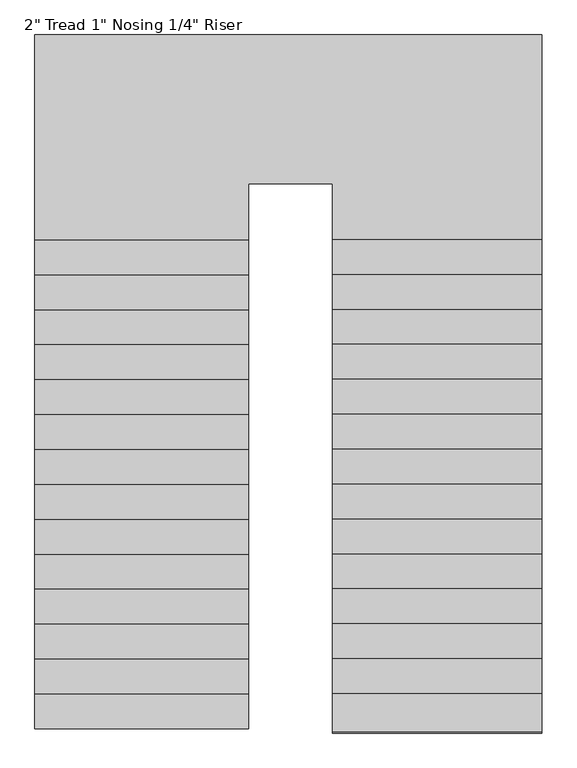
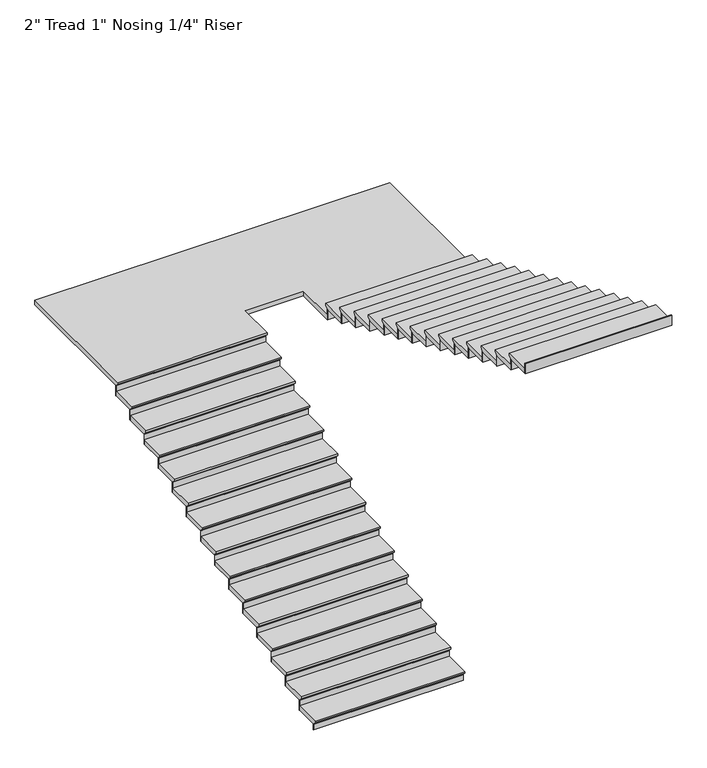
"""IFC4 building model written with IfcOpenShell, lengths in millimetres: stair flight geometry."""

from ifc_helpers import new_model, si_unit, origin, place, context, project, spatial, faceted_brep, source, transform, mapped, element, save


def stair_flight_0f889a08(model_context):
    return source(origin(), model_context, "Body", "Brep", [
        faceted_brep([(-5999.9290366, -6973.0610642, 8931.91), (-5999.9290366, -6973.0610642, 8950.96), (-7554.4415084, -6973.0610642, 8950.96), (-7554.4415084, -6973.0610642, 8931.91), (-5999.9290366, -6947.6610642, 8906.51), (-7554.4415084, -6947.6610642, 8906.51), (-5999.9290366, -6693.6610642, 8950.96), (-7554.4415084, -6693.6610642, 8950.96), (-7554.4415084, -6947.6610642, 8900.16), (-7554.4415084, -6693.6610642, 8900.16), (-5999.9290366, -6693.6610642, 8900.16), (-5999.9290366, -6947.6610642, 8900.16)], [[[0, 1, 2, 3]], [[4, 0, 3, 5]], [[2, 1, 6, 7]], [[8, 9, 10, 11]], [[2, 7, 9, 8, 5, 3]], [[8, 11, 4, 5]], [[6, 1, 0, 4, 11, 10]], [[7, 6, 10, 9]]]),
        faceted_brep([(-5999.9290366, -6947.6610642, 8900.16), (-5999.9290366, -6947.6610642, 8839.2), (-5999.9290366, -6941.3110642, 8839.2), (-5999.9290366, -6941.3110642, 8900.16), (-7554.4415084, -6947.6610642, 8900.16), (-7554.4415084, -6941.3110642, 8900.16), (-7554.4415084, -6941.3110642, 8839.2), (-7554.4415084, -6947.6610642, 8839.2)], [[[0, 1, 2, 3]], [[4, 5, 6, 7]], [[1, 0, 4, 7]], [[2, 1, 7, 6]], [[3, 2, 6, 5]], [[0, 3, 5, 4]]]),
        faceted_brep([(-5999.9290366, -6693.6610642, 9011.92), (-5999.9290366, -6693.6610642, 8900.16), (-5999.9290366, -6687.3110642, 8900.16), (-5999.9290366, -6687.3110642, 9011.92), (-7554.4415084, -6693.6610642, 9011.92), (-7554.4415084, -6687.3110642, 9011.92), (-7554.4415084, -6687.3110642, 8900.16), (-7554.4415084, -6693.6610642, 8900.16)], [[[0, 1, 2, 3]], [[4, 5, 6, 7]], [[1, 0, 4, 7]], [[2, 1, 7, 6]], [[3, 2, 6, 5]], [[0, 3, 5, 4]]]),
        faceted_brep([(-7554.4415084, -6719.0610642, 9062.72), (-5999.9290366, -6719.0610642, 9062.72), (-5999.9290366, -6439.6610642, 9062.72), (-7554.4415084, -6439.6610642, 9062.72), (-7554.4415084, -6693.6610642, 9011.92), (-7554.4415084, -6439.6610642, 9011.92), (-5999.9290366, -6439.6610642, 9011.92), (-5999.9290366, -6693.6610642, 9011.92), (-7554.4415084, -6693.6610642, 9018.27), (-7554.4415084, -6719.0610642, 9043.67), (-5999.9290366, -6693.6610642, 9018.27), (-5999.9290366, -6719.0610642, 9043.67)], [[[0, 1, 2, 3]], [[4, 5, 6, 7]], [[0, 3, 5, 4, 8, 9]], [[4, 7, 10, 8]], [[2, 1, 11, 10, 7, 6]], [[3, 2, 6, 5]], [[11, 1, 0, 9]], [[10, 11, 9, 8]]]),
        faceted_brep([(-5999.9290366, -6439.6610642, 9123.68), (-5999.9290366, -6439.6610642, 9011.92), (-5999.9290366, -6433.3110642, 9011.92), (-5999.9290366, -6433.3110642, 9123.68), (-7554.4415084, -6439.6610642, 9123.68), (-7554.4415084, -6433.3110642, 9123.68), (-7554.4415084, -6433.3110642, 9011.92), (-7554.4415084, -6439.6610642, 9011.92)], [[[0, 1, 2, 3]], [[4, 5, 6, 7]], [[1, 0, 4, 7]], [[2, 1, 7, 6]], [[3, 2, 6, 5]], [[0, 3, 5, 4]]]),
        faceted_brep([(-7554.4415084, -6465.0610642, 9174.48), (-5999.9290366, -6465.0610642, 9174.48), (-5999.9290366, -6185.6610642, 9174.48), (-7554.4415084, -6185.6610642, 9174.48), (-7554.4415084, -6439.6610642, 9123.68), (-7554.4415084, -6185.6610642, 9123.68), (-5999.9290366, -6185.6610642, 9123.68), (-5999.9290366, -6439.6610642, 9123.68), (-7554.4415084, -6439.6610642, 9130.03), (-7554.4415084, -6465.0610642, 9155.43), (-5999.9290366, -6439.6610642, 9130.03), (-5999.9290366, -6465.0610642, 9155.43)], [[[0, 1, 2, 3]], [[4, 5, 6, 7]], [[0, 3, 5, 4, 8, 9]], [[4, 7, 10, 8]], [[2, 1, 11, 10, 7, 6]], [[3, 2, 6, 5]], [[11, 1, 0, 9]], [[10, 11, 9, 8]]]),
        faceted_brep([(-5999.9290366, -6185.6610642, 9235.44), (-5999.9290366, -6185.6610642, 9123.68), (-5999.9290366, -6179.3110642, 9123.68), (-5999.9290366, -6179.3110642, 9235.44), (-7554.4415084, -6185.6610642, 9235.44), (-7554.4415084, -6179.3110642, 9235.44), (-7554.4415084, -6179.3110642, 9123.68), (-7554.4415084, -6185.6610642, 9123.68)], [[[0, 1, 2, 3]], [[4, 5, 6, 7]], [[1, 0, 4, 7]], [[2, 1, 7, 6]], [[3, 2, 6, 5]], [[0, 3, 5, 4]]]),
        faceted_brep([(-7554.4415084, -6211.0610642, 9286.24), (-5999.9290366, -6211.0610642, 9286.24), (-5999.9290366, -5931.6610642, 9286.24), (-7554.4415084, -5931.6610642, 9286.24), (-7554.4415084, -6185.6610642, 9235.44), (-7554.4415084, -5931.6610642, 9235.44), (-5999.9290366, -5931.6610642, 9235.44), (-5999.9290366, -6185.6610642, 9235.44), (-7554.4415084, -6185.6610642, 9241.79), (-7554.4415084, -6211.0610642, 9267.19), (-5999.9290366, -6185.6610642, 9241.79), (-5999.9290366, -6211.0610642, 9267.19)], [[[0, 1, 2, 3]], [[4, 5, 6, 7]], [[0, 3, 5, 4, 8, 9]], [[4, 7, 10, 8]], [[2, 1, 11, 10, 7, 6]], [[3, 2, 6, 5]], [[11, 1, 0, 9]], [[10, 11, 9, 8]]]),
        faceted_brep([(-5999.9290366, -5931.6610642, 9347.2), (-5999.9290366, -5931.6610642, 9235.44), (-5999.9290366, -5925.3110642, 9235.44), (-5999.9290366, -5925.3110642, 9347.2), (-7554.4415084, -5931.6610642, 9347.2), (-7554.4415084, -5925.3110642, 9347.2), (-7554.4415084, -5925.3110642, 9235.44), (-7554.4415084, -5931.6610642, 9235.44)], [[[0, 1, 2, 3]], [[4, 5, 6, 7]], [[1, 0, 4, 7]], [[2, 1, 7, 6]], [[3, 2, 6, 5]], [[0, 3, 5, 4]]]),
        faceted_brep([(-7554.4415084, -5957.0610642, 9398.0), (-5999.9290366, -5957.0610642, 9398.0), (-5999.9290366, -5677.6610642, 9398.0), (-7554.4415084, -5677.6610642, 9398.0), (-7554.4415084, -5931.6610642, 9347.2), (-7554.4415084, -5677.6610642, 9347.2), (-5999.9290366, -5677.6610642, 9347.2), (-5999.9290366, -5931.6610642, 9347.2), (-7554.4415084, -5931.6610642, 9353.55), (-7554.4415084, -5957.0610642, 9378.95), (-5999.9290366, -5931.6610642, 9353.55), (-5999.9290366, -5957.0610642, 9378.95)], [[[0, 1, 2, 3]], [[4, 5, 6, 7]], [[0, 3, 5, 4, 8, 9]], [[4, 7, 10, 8]], [[2, 1, 11, 10, 7, 6]], [[3, 2, 6, 5]], [[11, 1, 0, 9]], [[10, 11, 9, 8]]]),
        faceted_brep([(-5999.9290366, -5677.6610642, 9458.96), (-5999.9290366, -5677.6610642, 9347.2), (-5999.9290366, -5671.3110642, 9347.2), (-5999.9290366, -5671.3110642, 9458.96), (-7554.4415084, -5677.6610642, 9458.96), (-7554.4415084, -5671.3110642, 9458.96), (-7554.4415084, -5671.3110642, 9347.2), (-7554.4415084, -5677.6610642, 9347.2)], [[[0, 1, 2, 3]], [[4, 5, 6, 7]], [[1, 0, 4, 7]], [[2, 1, 7, 6]], [[3, 2, 6, 5]], [[0, 3, 5, 4]]]),
        faceted_brep([(-7554.4415084, -5703.0610642, 9509.76), (-5999.9290366, -5703.0610642, 9509.76), (-5999.9290366, -5423.6610642, 9509.76), (-7554.4415084, -5423.6610642, 9509.76), (-7554.4415084, -5677.6610642, 9458.96), (-7554.4415084, -5423.6610642, 9458.96), (-5999.9290366, -5423.6610642, 9458.96), (-5999.9290366, -5677.6610642, 9458.96), (-7554.4415084, -5677.6610642, 9465.31), (-7554.4415084, -5703.0610642, 9490.71), (-5999.9290366, -5677.6610642, 9465.31), (-5999.9290366, -5703.0610642, 9490.71)], [[[0, 1, 2, 3]], [[4, 5, 6, 7]], [[0, 3, 5, 4, 8, 9]], [[4, 7, 10, 8]], [[2, 1, 11, 10, 7, 6]], [[3, 2, 6, 5]], [[11, 1, 0, 9]], [[10, 11, 9, 8]]]),
        faceted_brep([(-5999.9290366, -5423.6610642, 9570.72), (-5999.9290366, -5423.6610642, 9458.96), (-5999.9290366, -5417.3110642, 9458.96), (-5999.9290366, -5417.3110642, 9570.72), (-7554.4415084, -5423.6610642, 9570.72), (-7554.4415084, -5417.3110642, 9570.72), (-7554.4415084, -5417.3110642, 9458.96), (-7554.4415084, -5423.6610642, 9458.96)], [[[0, 1, 2, 3]], [[4, 5, 6, 7]], [[1, 0, 4, 7]], [[2, 1, 7, 6]], [[3, 2, 6, 5]], [[0, 3, 5, 4]]]),
        faceted_brep([(-7554.4415084, -5449.0610642, 9621.52), (-5999.9290366, -5449.0610642, 9621.52), (-5999.9290366, -5169.6610642, 9621.52), (-7554.4415084, -5169.6610642, 9621.52), (-7554.4415084, -5423.6610642, 9570.72), (-7554.4415084, -5169.6610642, 9570.72), (-5999.9290366, -5169.6610642, 9570.72), (-5999.9290366, -5423.6610642, 9570.72), (-7554.4415084, -5423.6610642, 9577.07), (-7554.4415084, -5449.0610642, 9602.47), (-5999.9290366, -5423.6610642, 9577.07), (-5999.9290366, -5449.0610642, 9602.47)], [[[0, 1, 2, 3]], [[4, 5, 6, 7]], [[0, 3, 5, 4, 8, 9]], [[4, 7, 10, 8]], [[2, 1, 11, 10, 7, 6]], [[3, 2, 6, 5]], [[11, 1, 0, 9]], [[10, 11, 9, 8]]]),
        faceted_brep([(-5999.9290366, -5169.6610642, 9682.48), (-5999.9290366, -5169.6610642, 9570.72), (-5999.9290366, -5163.3110642, 9570.72), (-5999.9290366, -5163.3110642, 9682.48), (-7554.4415084, -5169.6610642, 9682.48), (-7554.4415084, -5163.3110642, 9682.48), (-7554.4415084, -5163.3110642, 9570.72), (-7554.4415084, -5169.6610642, 9570.72)], [[[0, 1, 2, 3]], [[4, 5, 6, 7]], [[1, 0, 4, 7]], [[2, 1, 7, 6]], [[3, 2, 6, 5]], [[0, 3, 5, 4]]]),
        faceted_brep([(-7554.4415084, -5195.0610642, 9733.28), (-5999.9290366, -5195.0610642, 9733.28), (-5999.9290366, -4915.6610642, 9733.28), (-7554.4415084, -4915.6610642, 9733.28), (-7554.4415084, -5169.6610642, 9682.48), (-7554.4415084, -4915.6610642, 9682.48), (-5999.9290366, -4915.6610642, 9682.48), (-5999.9290366, -5169.6610642, 9682.48), (-7554.4415084, -5169.6610642, 9688.83), (-7554.4415084, -5195.0610642, 9714.23), (-5999.9290366, -5169.6610642, 9688.83), (-5999.9290366, -5195.0610642, 9714.23)], [[[0, 1, 2, 3]], [[4, 5, 6, 7]], [[0, 3, 5, 4, 8, 9]], [[4, 7, 10, 8]], [[2, 1, 11, 10, 7, 6]], [[3, 2, 6, 5]], [[11, 1, 0, 9]], [[10, 11, 9, 8]]]),
        faceted_brep([(-5999.9290366, -4915.6610642, 9794.24), (-5999.9290366, -4915.6610642, 9682.48), (-5999.9290366, -4909.3110642, 9682.48), (-5999.9290366, -4909.3110642, 9794.24), (-7554.4415084, -4915.6610642, 9794.24), (-7554.4415084, -4909.3110642, 9794.24), (-7554.4415084, -4909.3110642, 9682.48), (-7554.4415084, -4915.6610642, 9682.48)], [[[0, 1, 2, 3]], [[4, 5, 6, 7]], [[1, 0, 4, 7]], [[2, 1, 7, 6]], [[3, 2, 6, 5]], [[0, 3, 5, 4]]]),
        faceted_brep([(-7554.4415084, -4941.0610642, 9845.04), (-5999.9290366, -4941.0610642, 9845.04), (-5999.9290366, -4661.6610642, 9845.04), (-7554.4415084, -4661.6610642, 9845.04), (-7554.4415084, -4915.6610642, 9794.24), (-7554.4415084, -4661.6610642, 9794.24), (-5999.9290366, -4661.6610642, 9794.24), (-5999.9290366, -4915.6610642, 9794.24), (-7554.4415084, -4915.6610642, 9800.59), (-7554.4415084, -4941.0610642, 9825.99), (-5999.9290366, -4915.6610642, 9800.59), (-5999.9290366, -4941.0610642, 9825.99)], [[[0, 1, 2, 3]], [[4, 5, 6, 7]], [[0, 3, 5, 4, 8, 9]], [[4, 7, 10, 8]], [[2, 1, 11, 10, 7, 6]], [[3, 2, 6, 5]], [[11, 1, 0, 9]], [[10, 11, 9, 8]]]),
        faceted_brep([(-5999.9290366, -4661.6610642, 9906.0), (-5999.9290366, -4661.6610642, 9794.24), (-5999.9290366, -4655.3110642, 9794.24), (-5999.9290366, -4655.3110642, 9906.0), (-7554.4415084, -4661.6610642, 9906.0), (-7554.4415084, -4655.3110642, 9906.0), (-7554.4415084, -4655.3110642, 9794.24), (-7554.4415084, -4661.6610642, 9794.24)], [[[0, 1, 2, 3]], [[4, 5, 6, 7]], [[1, 0, 4, 7]], [[2, 1, 7, 6]], [[3, 2, 6, 5]], [[0, 3, 5, 4]]]),
        faceted_brep([(-7554.4415084, -4687.0610642, 9956.8), (-5999.9290366, -4687.0610642, 9956.8), (-5999.9290366, -4407.6610642, 9956.8), (-7554.4415084, -4407.6610642, 9956.8), (-7554.4415084, -4661.6610642, 9906.0), (-7554.4415084, -4407.6610642, 9906.0), (-5999.9290366, -4407.6610642, 9906.0), (-5999.9290366, -4661.6610642, 9906.0), (-7554.4415084, -4661.6610642, 9912.35), (-7554.4415084, -4687.0610642, 9937.75), (-5999.9290366, -4661.6610642, 9912.35), (-5999.9290366, -4687.0610642, 9937.75)], [[[0, 1, 2, 3]], [[4, 5, 6, 7]], [[0, 3, 5, 4, 8, 9]], [[4, 7, 10, 8]], [[2, 1, 11, 10, 7, 6]], [[3, 2, 6, 5]], [[11, 1, 0, 9]], [[10, 11, 9, 8]]]),
        faceted_brep([(-5999.9290366, -4407.6610642, 10017.76), (-5999.9290366, -4407.6610642, 9906.0), (-5999.9290366, -4401.3110642, 9906.0), (-5999.9290366, -4401.3110642, 10017.76), (-7554.4415084, -4407.6610642, 10017.76), (-7554.4415084, -4401.3110642, 10017.76), (-7554.4415084, -4401.3110642, 9906.0), (-7554.4415084, -4407.6610642, 9906.0)], [[[0, 1, 2, 3]], [[4, 5, 6, 7]], [[1, 0, 4, 7]], [[2, 1, 7, 6]], [[3, 2, 6, 5]], [[0, 3, 5, 4]]]),
        faceted_brep([(-7554.4415084, -4433.0610642, 10068.56), (-5999.9290366, -4433.0610642, 10068.56), (-5999.9290366, -4153.6610642, 10068.56), (-7554.4415084, -4153.6610642, 10068.56), (-7554.4415084, -4407.6610642, 10017.76), (-7554.4415084, -4153.6610642, 10017.76), (-5999.9290366, -4153.6610642, 10017.76), (-5999.9290366, -4407.6610642, 10017.76), (-7554.4415084, -4407.6610642, 10024.11), (-7554.4415084, -4433.0610642, 10049.51), (-5999.9290366, -4407.6610642, 10024.11), (-5999.9290366, -4433.0610642, 10049.51)], [[[0, 1, 2, 3]], [[4, 5, 6, 7]], [[0, 3, 5, 4, 8, 9]], [[4, 7, 10, 8]], [[2, 1, 11, 10, 7, 6]], [[3, 2, 6, 5]], [[11, 1, 0, 9]], [[10, 11, 9, 8]]]),
        faceted_brep([(-5999.9290366, -4153.6610642, 10129.52), (-5999.9290366, -4153.6610642, 10017.76), (-5999.9290366, -4147.3110642, 10017.76), (-5999.9290366, -4147.3110642, 10129.52), (-7554.4415084, -4153.6610642, 10129.52), (-7554.4415084, -4147.3110642, 10129.52), (-7554.4415084, -4147.3110642, 10017.76), (-7554.4415084, -4153.6610642, 10017.76)], [[[0, 1, 2, 3]], [[4, 5, 6, 7]], [[1, 0, 4, 7]], [[2, 1, 7, 6]], [[3, 2, 6, 5]], [[0, 3, 5, 4]]]),
        faceted_brep([(-7554.4415084, -4179.0610642, 10180.32), (-5999.9290366, -4179.0610642, 10180.32), (-5999.9290366, -3899.6610642, 10180.32), (-7554.4415084, -3899.6610642, 10180.32), (-7554.4415084, -4153.6610642, 10129.52), (-7554.4415084, -3899.6610642, 10129.52), (-5999.9290366, -3899.6610642, 10129.52), (-5999.9290366, -4153.6610642, 10129.52), (-7554.4415084, -4153.6610642, 10135.87), (-7554.4415084, -4179.0610642, 10161.27), (-5999.9290366, -4153.6610642, 10135.87), (-5999.9290366, -4179.0610642, 10161.27)], [[[0, 1, 2, 3]], [[4, 5, 6, 7]], [[0, 3, 5, 4, 8, 9]], [[4, 7, 10, 8]], [[2, 1, 11, 10, 7, 6]], [[3, 2, 6, 5]], [[11, 1, 0, 9]], [[10, 11, 9, 8]]]),
        faceted_brep([(-5999.9290366, -3899.6610642, 10241.28), (-5999.9290366, -3899.6610642, 10129.52), (-5999.9290366, -3893.3110642, 10129.52), (-5999.9290366, -3893.3110642, 10241.28), (-7554.4415084, -3899.6610642, 10241.28), (-7554.4415084, -3893.3110642, 10241.28), (-7554.4415084, -3893.3110642, 10129.52), (-7554.4415084, -3899.6610642, 10129.52)], [[[0, 1, 2, 3]], [[4, 5, 6, 7]], [[1, 0, 4, 7]], [[2, 1, 7, 6]], [[3, 2, 6, 5]], [[0, 3, 5, 4]]]),
        faceted_brep([(-7554.4415084, -3925.0610642, 10292.08), (-5999.9290366, -3925.0610642, 10292.08), (-5999.9290366, -3645.6610642, 10292.08), (-7554.4415084, -3645.6610642, 10292.08), (-7554.4415084, -3899.6610642, 10241.28), (-7554.4415084, -3645.6610642, 10241.28), (-5999.9290366, -3645.6610642, 10241.28), (-5999.9290366, -3899.6610642, 10241.28), (-7554.4415084, -3899.6610642, 10247.63), (-7554.4415084, -3925.0610642, 10273.03), (-5999.9290366, -3899.6610642, 10247.63), (-5999.9290366, -3925.0610642, 10273.03)], [[[0, 1, 2, 3]], [[4, 5, 6, 7]], [[0, 3, 5, 4, 8, 9]], [[4, 7, 10, 8]], [[2, 1, 11, 10, 7, 6]], [[3, 2, 6, 5]], [[11, 1, 0, 9]], [[10, 11, 9, 8]]]),
        faceted_brep([(-5999.9290366, -3645.6610642, 10353.04), (-5999.9290366, -3645.6610642, 10241.28), (-5999.9290366, -3639.3110642, 10241.28), (-5999.9290366, -3639.3110642, 10353.04), (-7554.4415084, -3645.6610642, 10353.04), (-7554.4415084, -3639.3110642, 10353.04), (-7554.4415084, -3639.3110642, 10241.28), (-7554.4415084, -3645.6610642, 10241.28)], [[[0, 1, 2, 3]], [[4, 5, 6, 7]], [[1, 0, 4, 7]], [[2, 1, 7, 6]], [[3, 2, 6, 5]], [[0, 3, 5, 4]]]),
        faceted_brep([(-7554.4415084, -3671.0610642, 10403.84), (-5999.9290366, -3671.0610642, 10403.84), (-5999.9290366, -3391.6610642, 10403.84), (-7554.4415084, -3391.6610642, 10403.84), (-7554.4415084, -3645.6610642, 10353.04), (-7554.4415084, -3391.6610642, 10353.04), (-5999.9290366, -3391.6610642, 10353.04), (-5999.9290366, -3645.6610642, 10353.04), (-7554.4415084, -3645.6610642, 10359.39), (-7554.4415084, -3671.0610642, 10384.79), (-5999.9290366, -3645.6610642, 10359.39), (-5999.9290366, -3671.0610642, 10384.79)], [[[0, 1, 2, 3]], [[4, 5, 6, 7]], [[0, 3, 5, 4, 8, 9]], [[4, 7, 10, 8]], [[2, 1, 11, 10, 7, 6]], [[3, 2, 6, 5]], [[11, 1, 0, 9]], [[10, 11, 9, 8]]]),
        faceted_brep([(-5999.9290366, -3391.6610642, 10464.8), (-5999.9290366, -3391.6610642, 10353.04), (-5999.9290366, -3385.3110642, 10353.04), (-5999.9290366, -3385.3110642, 10464.8), (-7554.4415084, -3391.6610642, 10464.8), (-7554.4415084, -3385.3110642, 10464.8), (-7554.4415084, -3385.3110642, 10353.04), (-7554.4415084, -3391.6610642, 10353.04)], [[[0, 1, 2, 3]], [[4, 5, 6, 7]], [[1, 0, 4, 7]], [[2, 1, 7, 6]], [[3, 2, 6, 5]], [[0, 3, 5, 4]]]),
        faceted_brep([(-3866.3290366, -3442.4610642, 10515.6), (-3866.3290366, -1928.4217109, 10515.6), (-7554.4415084, -1928.4217109, 10515.6), (-7554.4415084, -3417.0610642, 10515.6), (-5999.9290366, -3417.0610642, 10515.6), (-5999.9290366, -3010.6610642, 10515.6), (-5390.3290366, -3010.6610642, 10515.6), (-5390.3290366, -3442.4610642, 10515.6), (-3866.3290366, -1928.4217109, 10464.8), (-3866.3290366, -3442.4610642, 10464.8), (-5390.3290366, -3442.4610642, 10464.8), (-5390.3290366, -3010.6610642, 10464.8), (-5999.9290366, -3010.6610642, 10464.8), (-5999.9290366, -3391.6610642, 10464.8), (-7554.4415084, -3391.6610642, 10464.8), (-7554.4415084, -1928.4217109, 10464.8), (-7554.4415084, -3391.6610642, 10471.15), (-7554.4415084, -3417.0610642, 10496.55), (-5999.9290366, -3391.6610642, 10471.15), (-5999.9290366, -3417.0610642, 10496.55)], [[[0, 1, 2, 3, 4, 5, 6, 7]], [[8, 9, 10, 11, 12, 13, 14, 15]], [[1, 0, 9, 8]], [[2, 1, 8, 15]], [[3, 2, 15, 14, 16, 17]], [[14, 13, 18, 16]], [[5, 4, 19, 18, 13, 12]], [[6, 5, 12, 11]], [[7, 6, 11, 10]], [[0, 7, 10, 9]], [[19, 4, 3, 17]], [[18, 19, 17, 16]]]),
        faceted_brep([(-5390.3290366, -3442.4610642, 10576.56), (-5390.3290366, -3442.4610642, 10464.8), (-5390.3290366, -3448.8110642, 10464.8), (-5390.3290366, -3448.8110642, 10576.56), (-3866.3290366, -3442.4610642, 10576.56), (-3866.3290366, -3448.8110642, 10576.56), (-3866.3290366, -3448.8110642, 10464.8), (-3866.3290366, -3442.4610642, 10464.8)], [[[0, 1, 2, 3]], [[4, 5, 6, 7]], [[1, 0, 4, 7]], [[2, 1, 7, 6]], [[3, 2, 6, 5]], [[0, 3, 5, 4]]]),
        faceted_brep([(-3866.3290366, -3417.0610642, 10627.36), (-5390.3290366, -3417.0610642, 10627.36), (-5390.3290366, -3696.4610642, 10627.36), (-3866.3290366, -3696.4610642, 10627.36), (-3866.3290366, -3442.4610642, 10576.56), (-3866.3290366, -3696.4610642, 10576.56), (-5390.3290366, -3696.4610642, 10576.56), (-5390.3290366, -3442.4610642, 10576.56), (-3866.3290366, -3442.4610642, 10582.91), (-3866.3290366, -3417.0610642, 10608.31), (-5390.3290366, -3442.4610642, 10582.91), (-5390.3290366, -3417.0610642, 10608.31)], [[[0, 1, 2, 3]], [[4, 5, 6, 7]], [[0, 3, 5, 4, 8, 9]], [[4, 7, 10, 8]], [[2, 1, 11, 10, 7, 6]], [[3, 2, 6, 5]], [[11, 1, 0, 9]], [[10, 11, 9, 8]]]),
        faceted_brep([(-5390.3290366, -3696.4610642, 10688.32), (-5390.3290366, -3696.4610642, 10576.56), (-5390.3290366, -3702.8110642, 10576.56), (-5390.3290366, -3702.8110642, 10688.32), (-3866.3290366, -3696.4610642, 10688.32), (-3866.3290366, -3702.8110642, 10688.32), (-3866.3290366, -3702.8110642, 10576.56), (-3866.3290366, -3696.4610642, 10576.56)], [[[0, 1, 2, 3]], [[4, 5, 6, 7]], [[1, 0, 4, 7]], [[2, 1, 7, 6]], [[3, 2, 6, 5]], [[0, 3, 5, 4]]]),
        faceted_brep([(-3866.3290366, -3671.0610642, 10739.12), (-5390.3290366, -3671.0610642, 10739.12), (-5390.3290366, -3950.4610642, 10739.12), (-3866.3290366, -3950.4610642, 10739.12), (-3866.3290366, -3696.4610642, 10688.32), (-3866.3290366, -3950.4610642, 10688.32), (-5390.3290366, -3950.4610642, 10688.32), (-5390.3290366, -3696.4610642, 10688.32), (-3866.3290366, -3696.4610642, 10694.67), (-3866.3290366, -3671.0610642, 10720.07), (-5390.3290366, -3696.4610642, 10694.67), (-5390.3290366, -3671.0610642, 10720.07)], [[[0, 1, 2, 3]], [[4, 5, 6, 7]], [[0, 3, 5, 4, 8, 9]], [[4, 7, 10, 8]], [[2, 1, 11, 10, 7, 6]], [[3, 2, 6, 5]], [[11, 1, 0, 9]], [[10, 11, 9, 8]]]),
        faceted_brep([(-5390.3290366, -3950.4610642, 10800.08), (-5390.3290366, -3950.4610642, 10688.32), (-5390.3290366, -3956.8110642, 10688.32), (-5390.3290366, -3956.8110642, 10800.08), (-3866.3290366, -3950.4610642, 10800.08), (-3866.3290366, -3956.8110642, 10800.08), (-3866.3290366, -3956.8110642, 10688.32), (-3866.3290366, -3950.4610642, 10688.32)], [[[0, 1, 2, 3]], [[4, 5, 6, 7]], [[1, 0, 4, 7]], [[2, 1, 7, 6]], [[3, 2, 6, 5]], [[0, 3, 5, 4]]]),
        faceted_brep([(-3866.3290366, -3925.0610642, 10850.88), (-5390.3290366, -3925.0610642, 10850.88), (-5390.3290366, -4204.4610642, 10850.88), (-3866.3290366, -4204.4610642, 10850.88), (-3866.3290366, -3950.4610642, 10800.08), (-3866.3290366, -4204.4610642, 10800.08), (-5390.3290366, -4204.4610642, 10800.08), (-5390.3290366, -3950.4610642, 10800.08), (-3866.3290366, -3950.4610642, 10806.43), (-3866.3290366, -3925.0610642, 10831.83), (-5390.3290366, -3950.4610642, 10806.43), (-5390.3290366, -3925.0610642, 10831.83)], [[[0, 1, 2, 3]], [[4, 5, 6, 7]], [[0, 3, 5, 4, 8, 9]], [[4, 7, 10, 8]], [[2, 1, 11, 10, 7, 6]], [[3, 2, 6, 5]], [[11, 1, 0, 9]], [[10, 11, 9, 8]]]),
        faceted_brep([(-5390.3290366, -4204.4610642, 10911.84), (-5390.3290366, -4204.4610642, 10800.08), (-5390.3290366, -4210.8110642, 10800.08), (-5390.3290366, -4210.8110642, 10911.84), (-3866.3290366, -4204.4610642, 10911.84), (-3866.3290366, -4210.8110642, 10911.84), (-3866.3290366, -4210.8110642, 10800.08), (-3866.3290366, -4204.4610642, 10800.08)], [[[0, 1, 2, 3]], [[4, 5, 6, 7]], [[1, 0, 4, 7]], [[2, 1, 7, 6]], [[3, 2, 6, 5]], [[0, 3, 5, 4]]]),
        faceted_brep([(-3866.3290366, -4179.0610642, 10962.64), (-5390.3290366, -4179.0610642, 10962.64), (-5390.3290366, -4458.4610642, 10962.64), (-3866.3290366, -4458.4610642, 10962.64), (-3866.3290366, -4204.4610642, 10911.84), (-3866.3290366, -4458.4610642, 10911.84), (-5390.3290366, -4458.4610642, 10911.84), (-5390.3290366, -4204.4610642, 10911.84), (-3866.3290366, -4204.4610642, 10918.19), (-3866.3290366, -4179.0610642, 10943.59), (-5390.3290366, -4204.4610642, 10918.19), (-5390.3290366, -4179.0610642, 10943.59)], [[[0, 1, 2, 3]], [[4, 5, 6, 7]], [[0, 3, 5, 4, 8, 9]], [[4, 7, 10, 8]], [[2, 1, 11, 10, 7, 6]], [[3, 2, 6, 5]], [[11, 1, 0, 9]], [[10, 11, 9, 8]]]),
        faceted_brep([(-5390.3290366, -4458.4610642, 11023.6), (-5390.3290366, -4458.4610642, 10911.84), (-5390.3290366, -4464.8110642, 10911.84), (-5390.3290366, -4464.8110642, 11023.6), (-3866.3290366, -4458.4610642, 11023.6), (-3866.3290366, -4464.8110642, 11023.6), (-3866.3290366, -4464.8110642, 10911.84), (-3866.3290366, -4458.4610642, 10911.84)], [[[0, 1, 2, 3]], [[4, 5, 6, 7]], [[1, 0, 4, 7]], [[2, 1, 7, 6]], [[3, 2, 6, 5]], [[0, 3, 5, 4]]]),
        faceted_brep([(-3866.3290366, -4433.0610642, 11074.4), (-5390.3290366, -4433.0610642, 11074.4), (-5390.3290366, -4712.4610642, 11074.4), (-3866.3290366, -4712.4610642, 11074.4), (-3866.3290366, -4458.4610642, 11023.6), (-3866.3290366, -4712.4610642, 11023.6), (-5390.3290366, -4712.4610642, 11023.6), (-5390.3290366, -4458.4610642, 11023.6), (-3866.3290366, -4458.4610642, 11029.95), (-3866.3290366, -4433.0610642, 11055.35), (-5390.3290366, -4458.4610642, 11029.95), (-5390.3290366, -4433.0610642, 11055.35)], [[[0, 1, 2, 3]], [[4, 5, 6, 7]], [[0, 3, 5, 4, 8, 9]], [[4, 7, 10, 8]], [[2, 1, 11, 10, 7, 6]], [[3, 2, 6, 5]], [[11, 1, 0, 9]], [[10, 11, 9, 8]]]),
        faceted_brep([(-5390.3290366, -4712.4610642, 11135.36), (-5390.3290366, -4712.4610642, 11023.6), (-5390.3290366, -4718.8110642, 11023.6), (-5390.3290366, -4718.8110642, 11135.36), (-3866.3290366, -4712.4610642, 11135.36), (-3866.3290366, -4718.8110642, 11135.36), (-3866.3290366, -4718.8110642, 11023.6), (-3866.3290366, -4712.4610642, 11023.6)], [[[0, 1, 2, 3]], [[4, 5, 6, 7]], [[1, 0, 4, 7]], [[2, 1, 7, 6]], [[3, 2, 6, 5]], [[0, 3, 5, 4]]]),
        faceted_brep([(-3866.3290366, -4687.0610642, 11186.16), (-5390.3290366, -4687.0610642, 11186.16), (-5390.3290366, -4966.4610642, 11186.16), (-3866.3290366, -4966.4610642, 11186.16), (-3866.3290366, -4712.4610642, 11135.36), (-3866.3290366, -4966.4610642, 11135.36), (-5390.3290366, -4966.4610642, 11135.36), (-5390.3290366, -4712.4610642, 11135.36), (-3866.3290366, -4712.4610642, 11141.71), (-3866.3290366, -4687.0610642, 11167.11), (-5390.3290366, -4712.4610642, 11141.71), (-5390.3290366, -4687.0610642, 11167.11)], [[[0, 1, 2, 3]], [[4, 5, 6, 7]], [[0, 3, 5, 4, 8, 9]], [[4, 7, 10, 8]], [[2, 1, 11, 10, 7, 6]], [[3, 2, 6, 5]], [[11, 1, 0, 9]], [[10, 11, 9, 8]]]),
        faceted_brep([(-5390.3290366, -4966.4610642, 11247.12), (-5390.3290366, -4966.4610642, 11135.36), (-5390.3290366, -4972.8110642, 11135.36), (-5390.3290366, -4972.8110642, 11247.12), (-3866.3290366, -4966.4610642, 11247.12), (-3866.3290366, -4972.8110642, 11247.12), (-3866.3290366, -4972.8110642, 11135.36), (-3866.3290366, -4966.4610642, 11135.36)], [[[0, 1, 2, 3]], [[4, 5, 6, 7]], [[1, 0, 4, 7]], [[2, 1, 7, 6]], [[3, 2, 6, 5]], [[0, 3, 5, 4]]]),
        faceted_brep([(-3866.3290366, -4941.0610642, 11297.92), (-5390.3290366, -4941.0610642, 11297.92), (-5390.3290366, -5220.4610642, 11297.92), (-3866.3290366, -5220.4610642, 11297.92), (-3866.3290366, -4966.4610642, 11247.12), (-3866.3290366, -5220.4610642, 11247.12), (-5390.3290366, -5220.4610642, 11247.12), (-5390.3290366, -4966.4610642, 11247.12), (-3866.3290366, -4966.4610642, 11253.47), (-3866.3290366, -4941.0610642, 11278.87), (-5390.3290366, -4966.4610642, 11253.47), (-5390.3290366, -4941.0610642, 11278.87)], [[[0, 1, 2, 3]], [[4, 5, 6, 7]], [[0, 3, 5, 4, 8, 9]], [[4, 7, 10, 8]], [[2, 1, 11, 10, 7, 6]], [[3, 2, 6, 5]], [[11, 1, 0, 9]], [[10, 11, 9, 8]]]),
        faceted_brep([(-5390.3290366, -5220.4610642, 11358.88), (-5390.3290366, -5220.4610642, 11247.12), (-5390.3290366, -5226.8110642, 11247.12), (-5390.3290366, -5226.8110642, 11358.88), (-3866.3290366, -5220.4610642, 11358.88), (-3866.3290366, -5226.8110642, 11358.88), (-3866.3290366, -5226.8110642, 11247.12), (-3866.3290366, -5220.4610642, 11247.12)], [[[0, 1, 2, 3]], [[4, 5, 6, 7]], [[1, 0, 4, 7]], [[2, 1, 7, 6]], [[3, 2, 6, 5]], [[0, 3, 5, 4]]]),
        faceted_brep([(-3866.3290366, -5195.0610642, 11409.68), (-5390.3290366, -5195.0610642, 11409.68), (-5390.3290366, -5474.4610642, 11409.68), (-3866.3290366, -5474.4610642, 11409.68), (-3866.3290366, -5220.4610642, 11358.88), (-3866.3290366, -5474.4610642, 11358.88), (-5390.3290366, -5474.4610642, 11358.88), (-5390.3290366, -5220.4610642, 11358.88), (-3866.3290366, -5220.4610642, 11365.23), (-3866.3290366, -5195.0610642, 11390.63), (-5390.3290366, -5220.4610642, 11365.23), (-5390.3290366, -5195.0610642, 11390.63)], [[[0, 1, 2, 3]], [[4, 5, 6, 7]], [[0, 3, 5, 4, 8, 9]], [[4, 7, 10, 8]], [[2, 1, 11, 10, 7, 6]], [[3, 2, 6, 5]], [[11, 1, 0, 9]], [[10, 11, 9, 8]]]),
        faceted_brep([(-5390.3290366, -5474.4610642, 11470.64), (-5390.3290366, -5474.4610642, 11358.88), (-5390.3290366, -5480.8110642, 11358.88), (-5390.3290366, -5480.8110642, 11470.64), (-3866.3290366, -5474.4610642, 11470.64), (-3866.3290366, -5480.8110642, 11470.64), (-3866.3290366, -5480.8110642, 11358.88), (-3866.3290366, -5474.4610642, 11358.88)], [[[0, 1, 2, 3]], [[4, 5, 6, 7]], [[1, 0, 4, 7]], [[2, 1, 7, 6]], [[3, 2, 6, 5]], [[0, 3, 5, 4]]]),
        faceted_brep([(-3866.3290366, -5449.0610642, 11521.44), (-5390.3290366, -5449.0610642, 11521.44), (-5390.3290366, -5728.4610642, 11521.44), (-3866.3290366, -5728.4610642, 11521.44), (-3866.3290366, -5474.4610642, 11470.64), (-3866.3290366, -5728.4610642, 11470.64), (-5390.3290366, -5728.4610642, 11470.64), (-5390.3290366, -5474.4610642, 11470.64), (-3866.3290366, -5474.4610642, 11476.99), (-3866.3290366, -5449.0610642, 11502.39), (-5390.3290366, -5474.4610642, 11476.99), (-5390.3290366, -5449.0610642, 11502.39)], [[[0, 1, 2, 3]], [[4, 5, 6, 7]], [[0, 3, 5, 4, 8, 9]], [[4, 7, 10, 8]], [[2, 1, 11, 10, 7, 6]], [[3, 2, 6, 5]], [[11, 1, 0, 9]], [[10, 11, 9, 8]]]),
        faceted_brep([(-5390.3290366, -5728.4610642, 11582.4), (-5390.3290366, -5728.4610642, 11470.64), (-5390.3290366, -5734.8110642, 11470.64), (-5390.3290366, -5734.8110642, 11582.4), (-3866.3290366, -5728.4610642, 11582.4), (-3866.3290366, -5734.8110642, 11582.4), (-3866.3290366, -5734.8110642, 11470.64), (-3866.3290366, -5728.4610642, 11470.64)], [[[0, 1, 2, 3]], [[4, 5, 6, 7]], [[1, 0, 4, 7]], [[2, 1, 7, 6]], [[3, 2, 6, 5]], [[0, 3, 5, 4]]]),
        faceted_brep([(-3866.3290366, -5703.0610642, 11633.2), (-5390.3290366, -5703.0610642, 11633.2), (-5390.3290366, -5982.4610642, 11633.2), (-3866.3290366, -5982.4610642, 11633.2), (-3866.3290366, -5728.4610642, 11582.4), (-3866.3290366, -5982.4610642, 11582.4), (-5390.3290366, -5982.4610642, 11582.4), (-5390.3290366, -5728.4610642, 11582.4), (-3866.3290366, -5728.4610642, 11588.75), (-3866.3290366, -5703.0610642, 11614.15), (-5390.3290366, -5728.4610642, 11588.75), (-5390.3290366, -5703.0610642, 11614.15)], [[[0, 1, 2, 3]], [[4, 5, 6, 7]], [[0, 3, 5, 4, 8, 9]], [[4, 7, 10, 8]], [[2, 1, 11, 10, 7, 6]], [[3, 2, 6, 5]], [[11, 1, 0, 9]], [[10, 11, 9, 8]]]),
        faceted_brep([(-5390.3290366, -5982.4610642, 11694.16), (-5390.3290366, -5982.4610642, 11582.4), (-5390.3290366, -5988.8110642, 11582.4), (-5390.3290366, -5988.8110642, 11694.16), (-3866.3290366, -5982.4610642, 11694.16), (-3866.3290366, -5988.8110642, 11694.16), (-3866.3290366, -5988.8110642, 11582.4), (-3866.3290366, -5982.4610642, 11582.4)], [[[0, 1, 2, 3]], [[4, 5, 6, 7]], [[1, 0, 4, 7]], [[2, 1, 7, 6]], [[3, 2, 6, 5]], [[0, 3, 5, 4]]]),
        faceted_brep([(-3866.3290366, -5957.0610642, 11744.96), (-5390.3290366, -5957.0610642, 11744.96), (-5390.3290366, -6236.4610642, 11744.96), (-3866.3290366, -6236.4610642, 11744.96), (-3866.3290366, -5982.4610642, 11694.16), (-3866.3290366, -6236.4610642, 11694.16), (-5390.3290366, -6236.4610642, 11694.16), (-5390.3290366, -5982.4610642, 11694.16), (-3866.3290366, -5982.4610642, 11700.51), (-3866.3290366, -5957.0610642, 11725.91), (-5390.3290366, -5982.4610642, 11700.51), (-5390.3290366, -5957.0610642, 11725.91)], [[[0, 1, 2, 3]], [[4, 5, 6, 7]], [[0, 3, 5, 4, 8, 9]], [[4, 7, 10, 8]], [[2, 1, 11, 10, 7, 6]], [[3, 2, 6, 5]], [[11, 1, 0, 9]], [[10, 11, 9, 8]]]),
        faceted_brep([(-5390.3290366, -6236.4610642, 11805.92), (-5390.3290366, -6236.4610642, 11694.16), (-5390.3290366, -6242.8110642, 11694.16), (-5390.3290366, -6242.8110642, 11805.92), (-3866.3290366, -6236.4610642, 11805.92), (-3866.3290366, -6242.8110642, 11805.92), (-3866.3290366, -6242.8110642, 11694.16), (-3866.3290366, -6236.4610642, 11694.16)], [[[0, 1, 2, 3]], [[4, 5, 6, 7]], [[1, 0, 4, 7]], [[2, 1, 7, 6]], [[3, 2, 6, 5]], [[0, 3, 5, 4]]]),
        faceted_brep([(-3866.3290366, -6211.0610642, 11856.72), (-5390.3290366, -6211.0610642, 11856.72), (-5390.3290366, -6490.4610642, 11856.72), (-3866.3290366, -6490.4610642, 11856.72), (-3866.3290366, -6236.4610642, 11805.92), (-3866.3290366, -6490.4610642, 11805.92), (-5390.3290366, -6490.4610642, 11805.92), (-5390.3290366, -6236.4610642, 11805.92), (-3866.3290366, -6236.4610642, 11812.27), (-3866.3290366, -6211.0610642, 11837.67), (-5390.3290366, -6236.4610642, 11812.27), (-5390.3290366, -6211.0610642, 11837.67)], [[[0, 1, 2, 3]], [[4, 5, 6, 7]], [[0, 3, 5, 4, 8, 9]], [[4, 7, 10, 8]], [[2, 1, 11, 10, 7, 6]], [[3, 2, 6, 5]], [[11, 1, 0, 9]], [[10, 11, 9, 8]]]),
        faceted_brep([(-5390.3290366, -6490.4610642, 11917.68), (-5390.3290366, -6490.4610642, 11805.92), (-5390.3290366, -6496.8110642, 11805.92), (-5390.3290366, -6496.8110642, 11917.68), (-3866.3290366, -6490.4610642, 11917.68), (-3866.3290366, -6496.8110642, 11917.68), (-3866.3290366, -6496.8110642, 11805.92), (-3866.3290366, -6490.4610642, 11805.92)], [[[0, 1, 2, 3]], [[4, 5, 6, 7]], [[1, 0, 4, 7]], [[2, 1, 7, 6]], [[3, 2, 6, 5]], [[0, 3, 5, 4]]]),
        faceted_brep([(-3866.3290366, -6465.0610642, 11968.48), (-5390.3290366, -6465.0610642, 11968.48), (-5390.3290366, -6744.4610642, 11968.48), (-3866.3290366, -6744.4610642, 11968.48), (-3866.3290366, -6490.4610642, 11917.68), (-3866.3290366, -6744.4610642, 11917.68), (-5390.3290366, -6744.4610642, 11917.68), (-5390.3290366, -6490.4610642, 11917.68), (-3866.3290366, -6490.4610642, 11924.03), (-3866.3290366, -6465.0610642, 11949.43), (-5390.3290366, -6490.4610642, 11924.03), (-5390.3290366, -6465.0610642, 11949.43)], [[[0, 1, 2, 3]], [[4, 5, 6, 7]], [[0, 3, 5, 4, 8, 9]], [[4, 7, 10, 8]], [[2, 1, 11, 10, 7, 6]], [[3, 2, 6, 5]], [[11, 1, 0, 9]], [[10, 11, 9, 8]]]),
        faceted_brep([(-5390.3290366, -6744.4610642, 12029.44), (-5390.3290366, -6744.4610642, 11917.68), (-5390.3290366, -6750.8110642, 11917.68), (-5390.3290366, -6750.8110642, 12029.44), (-3866.3290366, -6744.4610642, 12029.44), (-3866.3290366, -6750.8110642, 12029.44), (-3866.3290366, -6750.8110642, 11917.68), (-3866.3290366, -6744.4610642, 11917.68)], [[[0, 1, 2, 3]], [[4, 5, 6, 7]], [[1, 0, 4, 7]], [[2, 1, 7, 6]], [[3, 2, 6, 5]], [[0, 3, 5, 4]]]),
        faceted_brep([(-5390.3290366, -6998.4610642, 12141.2), (-5390.3290366, -6998.4610642, 12029.44), (-5390.3290366, -7004.8110642, 12029.44), (-5390.3290366, -7004.8110642, 12141.2), (-3866.3290366, -6998.4610642, 12141.2), (-3866.3290366, -7004.8110642, 12141.2), (-3866.3290366, -7004.8110642, 12029.44), (-3866.3290366, -6998.4610642, 12029.44)], [[[0, 1, 2, 3]], [[4, 5, 6, 7]], [[1, 0, 4, 7]], [[2, 1, 7, 6]], [[3, 2, 6, 5]], [[0, 3, 5, 4]]]),
        faceted_brep([(-3866.3290366, -6719.0610642, 12080.24), (-5390.3290366, -6719.0610642, 12080.24), (-5390.3290366, -6998.4610642, 12080.24), (-3866.3290366, -6998.4610642, 12080.24), (-3866.3290366, -6744.4610642, 12029.44), (-3866.3290366, -6998.4610642, 12029.44), (-5390.3290366, -6998.4610642, 12029.44), (-5390.3290366, -6744.4610642, 12029.44), (-3866.3290366, -6744.4610642, 12035.79), (-3866.3290366, -6719.0610642, 12061.19), (-5390.3290366, -6744.4610642, 12035.79), (-5390.3290366, -6719.0610642, 12061.19)], [[[0, 1, 2, 3]], [[4, 5, 6, 7]], [[0, 3, 5, 4, 8, 9]], [[4, 7, 10, 8]], [[2, 1, 11, 10, 7, 6]], [[3, 2, 6, 5]], [[11, 1, 0, 9]], [[10, 11, 9, 8]]]),
    ])


if __name__ == "__main__":
    model = new_model("IFC4")
    model_context = context("Model", 3, world=origin())
    ifc_project = project(units=[si_unit("LENGTHUNIT", "METRE", prefix="MILLI")], contexts=[model_context])
    site = spatial("IfcSite", under=ifc_project)
    building = spatial("IfcBuilding", under=site)
    placement = place(None, origin())
    stair_flight_shape = stair_flight_0f889a08(model_context)
    element("IfcStairFlight", 1, ObjectType="2\" Tread 1\" Nosing 1/4\" Riser", at=placement, inside=building, context=model_context, shape_type="MappedRepresentation", body=[
        mapped(stair_flight_shape, transform((0.0, 0.0, 0.0), x_axis=(1.0, 0.0, 0.0), y_axis=(0.0, 1.0, 0.0), z_axis=(0.0, 0.0, 1.0))),
    ])
    save(model, "model.ifc")
